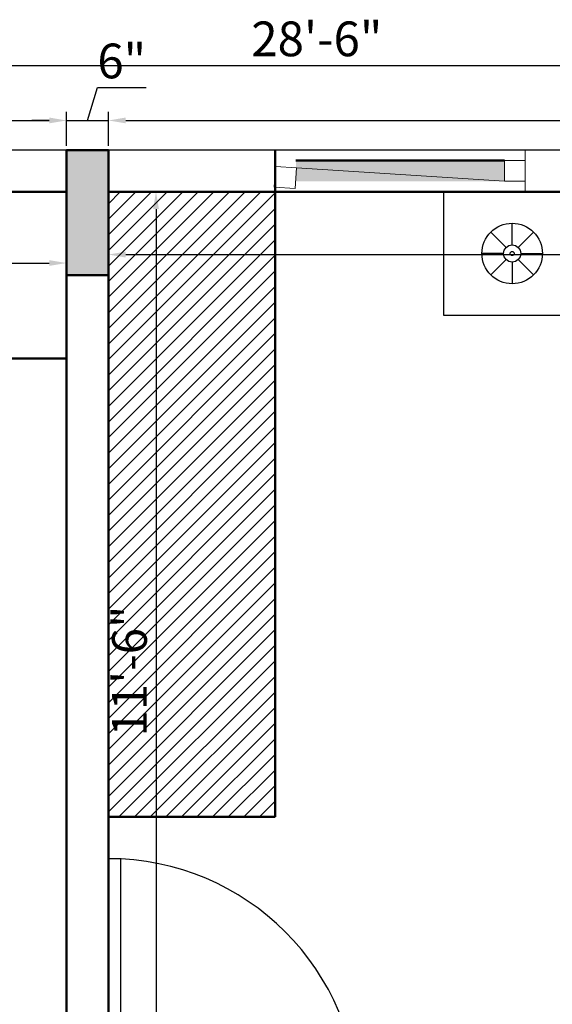
# Model space of a CAD drawing. Units: inches. Extents: x 3064 to 19385, y 846 to 15425.
# Tile 87 of 108: x 7228 to 7305, y 1273 to 1415. Entities that reach past the tile are written whole.
import ezdxf

# ---------------------------------------------------------------- set-up
doc = ezdxf.new("R2010")
doc.units = ezdxf.units.IN
for name, color, linetype, lineweight in [('A-ANNO-DIMS', 2, 'Continuous', 18), ('A-COLS', 1, 'Continuous', 35), ('A-DOOR', 3, 'Continuous', 25), ('A-FLOR-FIXT', 9, 'Continuous', 18), ('A-FURN-PATT', 252, 'Continuous', 13), ('A-GLAZ', 4, 'Continuous', 18), ('A-WALL', 7, 'Continuous', 50), ('C-PROP', 6, 'Continuous', 25)]:
    doc.layers.add(name, color=color, linetype=linetype, lineweight=lineweight)
doc.layers.add('BLOCK', color=6, linetype='Continuous')
doc.styles.get("Standard").update_dxf_attribs({"font": 'arial.ttf'})
doc.dimstyles.new('ISO-25', dxfattribs={"dimtxt": 9, "dimasz": 2.5, "dimexe": 1.25, "dimexo": 0.625, "dimtad": 1, "dimdec": 1, "dimlunit": 3, "dimtxsty": 'Standard', "dimcen": 2.5, "dimadec": 0, "dimazin": 0, "dimtfac": 1, "dimtdec": 1, "dimtmove": 0, "dimatfit": 3, "dimfxl": 1, "dimarcsym": 0})

# ---------------------------------------------------------------- blocks, each defined once
blk = doc.blocks.new('*U3')
for p, q in [((0, 0), (0, -6)), ((36, 0), (36, -6))]:
    blk.add_line(p, q)
blk.add_lwpolyline([(0, 0), (0, 36), (1.75, 36), (1.75, 0)], close=True)
blk.add_arc((0, 0), 36, 0, 90)
blk = doc.blocks.new('*D292')
at = {"layer": 'A-ANNO-DIMS', "color": 0, "lineweight": -2, "transparency": 16777216}
for p, q in [((7105.71, 1396.96), (7105.71, 1401.84)), ((7234.71, 1396.96), (7234.71, 1401.84)), ((7108.21, 1400.59), (7232.21, 1400.59))]:
    blk.add_line(p, q, dxfattribs=at)
at = {"layer": 'A-ANNO-DIMS', "color": 0, "transparency": 16777216}
for points in [[(7108.21, 1401.01), (7108.21, 1400.18), (7105.71, 1400.59)], [(7232.21, 1401.01), (7232.21, 1400.18), (7234.71, 1400.59)]]:
    blk.add_solid(points, dxfattribs=at)
at = {"layer": 'Defpoints', "color": 0, "transparency": 16777216}
for p in [(7234.71, 1400.59), (7105.71, 1396.34), (7234.71, 1396.34)]:
    blk.add_point(p, dxfattribs=at)
at = {"layer": 'A-ANNO-DIMS', "color": 0, "transparency": 16777216, "insert": (7170.21, 1403.77), "char_height": 5, "attachment_point": 5}
blk.add_mtext('10\'-9"', dxfattribs=at)
blk = doc.blocks.new('*D293')
at = {"layer": 'A-ANNO-DIMS', "color": 0, "lineweight": -2, "transparency": 16777216}
for p, q in [((7237.71, 1400.59), (7239.13, 1405.33)), ((7239.13, 1405.33), (7246.15, 1405.33)), ((7234.71, 1396.96), (7234.71, 1401.84)), ((7240.71, 1396.96), (7240.71, 1401.84)), ((7232.21, 1400.59), (7229.71, 1400.59)), ((7234.71, 1400.59), (7240.71, 1400.59)), ((7234.71, 1400.59), (7240.71, 1400.59)), ((7243.21, 1400.59), (7245.71, 1400.59))]:
    blk.add_line(p, q, dxfattribs=at)
at = {"layer": 'A-ANNO-DIMS', "color": 0, "transparency": 16777216}
for points in [[(7232.21, 1401.01), (7232.21, 1400.18), (7234.71, 1400.59)], [(7243.21, 1401.01), (7243.21, 1400.18), (7240.71, 1400.59)]]:
    blk.add_solid(points, dxfattribs=at)
at = {"layer": 'Defpoints', "color": 0, "transparency": 16777216}
for p in [(7240.71, 1400.59), (7234.71, 1396.34), (7240.71, 1396.34)]:
    blk.add_point(p, dxfattribs=at)
at = {"layer": 'A-ANNO-DIMS', "color": 0, "transparency": 16777216, "insert": (7242.64, 1408.51), "char_height": 5, "attachment_point": 5}
blk.add_mtext('6"', dxfattribs=at)
blk = doc.blocks.new('*D294')
at = {"layer": 'A-ANNO-DIMS', "color": 0, "lineweight": -2, "transparency": 16777216}
for p, q in [((7240.71, 1396.96), (7240.71, 1401.84)), ((7435.71, 1396.96), (7435.71, 1401.84)), ((7243.21, 1400.59), (7433.21, 1400.59))]:
    blk.add_line(p, q, dxfattribs=at)
at = {"layer": 'A-ANNO-DIMS', "color": 0, "transparency": 16777216}
for points in [[(7243.21, 1401.01), (7243.21, 1400.18), (7240.71, 1400.59)], [(7433.21, 1401.01), (7433.21, 1400.18), (7435.71, 1400.59)]]:
    blk.add_solid(points, dxfattribs=at)
at = {"layer": 'Defpoints', "color": 0, "transparency": 16777216}
for p in [(7435.71, 1400.59), (7240.71, 1396.34), (7435.71, 1396.34)]:
    blk.add_point(p, dxfattribs=at)
at = {"layer": 'A-ANNO-DIMS', "color": 0, "transparency": 16777216, "insert": (7338.21, 1403.77), "char_height": 5, "attachment_point": 5}
blk.add_mtext('16\'-3"', dxfattribs=at)
blk = doc.blocks.new('*D315')
at = {"layer": 'A-ANNO-DIMS', "color": 0, "lineweight": -2, "transparency": 16777216}
for p, q in [((7099.71, 1396.96), (7099.71, 1409.76)), ((7441.71, 1396.96), (7441.71, 1409.76)), ((7102.21, 1408.51), (7439.21, 1408.51))]:
    blk.add_line(p, q, dxfattribs=at)
at = {"layer": 'A-ANNO-DIMS', "color": 0, "transparency": 16777216}
for points in [[(7102.21, 1408.93), (7102.21, 1408.1), (7099.71, 1408.51)], [(7439.21, 1408.93), (7439.21, 1408.1), (7441.71, 1408.51)]]:
    blk.add_solid(points, dxfattribs=at)
at = {"layer": 'Defpoints', "color": 0, "transparency": 16777216}
for p in [(7441.71, 1408.51), (7099.71, 1396.34), (7441.71, 1396.34)]:
    blk.add_point(p, dxfattribs=at)
at = {"layer": 'A-ANNO-DIMS', "color": 0, "transparency": 16777216, "insert": (7270.71, 1411.69), "char_height": 5, "attachment_point": 5}
blk.add_mtext('28\'-6"', dxfattribs=at)
blk = doc.blocks.new('*D288')
at = {"layer": 'A-ANNO-DIMS', "color": 0, "lineweight": -2, "transparency": 16777216}
for p, q in [((7105.71, 1389.71), (7105.71, 1378.82)), ((7234.71, 1389.71), (7234.71, 1378.82)), ((7108.21, 1380.07), (7232.21, 1380.07))]:
    blk.add_line(p, q, dxfattribs=at)
at = {"layer": 'A-ANNO-DIMS', "color": 0, "transparency": 16777216}
for points in [[(7108.21, 1380.49), (7108.21, 1379.66), (7105.71, 1380.07)], [(7232.21, 1380.49), (7232.21, 1379.66), (7234.71, 1380.07)]]:
    blk.add_solid(points, dxfattribs=at)
at = {"layer": 'Defpoints', "color": 0, "transparency": 16777216}
for p in [(7105.71, 1390.34), (7234.71, 1390.34), (7234.71, 1380.07)]:
    blk.add_point(p, dxfattribs=at)
at = {"layer": 'A-ANNO-DIMS', "color": 0, "transparency": 16777216, "insert": (7170.21, 1383.25), "char_height": 5, "attachment_point": 5}
blk.add_mtext('10\'-9"', dxfattribs=at)
blk = doc.blocks.new('*D290')
at = {"layer": 'A-ANNO-DIMS', "color": 0, "lineweight": -2, "transparency": 16777216}
for p, q in [((7240.71, 1389.71), (7240.71, 1380.04)), ((7435.71, 1389.71), (7435.71, 1380.04)), ((7243.21, 1381.29), (7433.21, 1381.29))]:
    blk.add_line(p, q, dxfattribs=at)
at = {"layer": 'A-ANNO-DIMS', "color": 0, "transparency": 16777216}
for points in [[(7243.21, 1381.71), (7243.21, 1380.87), (7240.71, 1381.29)], [(7433.21, 1381.71), (7433.21, 1380.87), (7435.71, 1381.29)]]:
    blk.add_solid(points, dxfattribs=at)
at = {"layer": 'Defpoints', "color": 0, "transparency": 16777216}
for p in [(7240.71, 1390.34), (7435.71, 1390.34), (7435.71, 1381.29)]:
    blk.add_point(p, dxfattribs=at)
at = {"layer": 'A-ANNO-DIMS', "color": 0, "transparency": 16777216, "insert": (7338.21, 1384.47), "char_height": 5, "attachment_point": 5}
blk.add_mtext('16\'-3"', dxfattribs=at)
blk = doc.blocks.new('*D275')
at = {"layer": 'A-ANNO-DIMS', "color": 0, "lineweight": -2, "transparency": 16777216}
for p, q in [((7241.33, 1390.34), (7248.82, 1390.34)), ((7247.57, 1387.84), (7247.57, 1254.84)), ((7241.33, 1252.34), (7248.82, 1252.34))]:
    blk.add_line(p, q, dxfattribs=at)
at = {"layer": 'A-ANNO-DIMS', "color": 0, "transparency": 16777216}
for points in [[(7247.15, 1387.84), (7247.99, 1387.84), (7247.57, 1390.34)], [(7247.15, 1254.84), (7247.99, 1254.84), (7247.57, 1252.34)]]:
    blk.add_solid(points, dxfattribs=at)
at = {"layer": 'Defpoints', "color": 0, "transparency": 16777216}
for p in [(7240.71, 1390.34), (7240.71, 1252.34), (7247.57, 1252.34)]:
    blk.add_point(p, dxfattribs=at)
at = {"layer": 'A-ANNO-DIMS', "color": 0, "transparency": 16777216, "insert": (7244.39, 1321.34), "char_height": 5, "attachment_point": 5, "rotation": 90}
blk.add_mtext('11\'-6"', dxfattribs=at)
blk = doc.blocks.new('A$C52E67D0D')
at = {"layer": 'BLOCK'}
for p, q in [((250.5, 1605.5), (250.5, 1684.7)), ((228.3, 1596.3), (172.3, 1652.3)), ((272.7, 1596.3), (328.7, 1652.3)), ((219.1, 1574.1), (139.9, 1574.1)), ((228.3, 1551.9), (172.3, 1495.9)), ((272.7, 1551.9), (328.7, 1495.9)), ((281.9, 1574.1), (361.1, 1574.1)), ((250.5, 1542.8), (250.5, 1463.5))]:
    blk.add_line(p, q, dxfattribs=at)
blk.add_lwpolyline([(501, 1348.6), (501, 1799.6), (0, 1799.6), (0, 1348.6)], close=True, dxfattribs=at)
for radius in [110.6, 31.4, 7.46]:
    blk.add_circle((250.5, 1574.1), radius, dxfattribs=at)
blk = doc.blocks.new('WIN-900')
blk.add_line((0, 0), (30, 0))
blk.add_lwpolyline([(30, 0), (30, 3), (33, 3), (33, 0)], close=True)

msp = doc.modelspace()

# ---------------------------------------------------------------- hatches: boundary and pattern name
at = {"layer": 'A-COLS'}
h = msp.add_hatch(color=256, dxfattribs=at)
h.dxf.hatch_style = 1
h.paths.add_polyline_path([(7234.71, 1378.34), (7240.71, 1378.34), (7240.71, 1396.34), (7234.71, 1396.34)])
at = {"layer": 'A-FURN-PATT'}
h = msp.add_hatch(dxfattribs=at)
h.set_pattern_fill('ANSI31', color=256, scale=0.5)
h.set_pattern_definition([(45, (1784.0376, -1e-11), (-1.122532, 1.122532), [])])
h.paths.add_polyline_path([(7264.71, 1390.34), (7240.71, 1390.34), (7240.71, 1378.34), (7240.71, 1300.34), (7264.71, 1300.34)])
at = {"layer": 'A-GLAZ'}
h = msp.add_hatch(color=256, dxfattribs=at)
h.dxf.hatch_style = 1
h.paths.add_polyline_path([(7297.71, 1394.84), (7267.71, 1394.84), (7267.71, 1391.84), (7297.71, 1391.84)])

# ---------------------------------------------------------------- linework, layer by layer
msp.add_line((7300.71, 1396.34), (7300.71, 1390.34), dxfattribs=at)
msp.add_lwpolyline([(7300.71, 1391.84), (7297.71, 1391.84), (7297.71, 1394.84), (7300.71, 1394.84)], close=True, dxfattribs=at)
at = {"layer": 'A-WALL'}
for p, q in [((7264.71, 1396.34), (7264.71, 1390.34)), ((7267.71, 1394.84), (7297.71, 1394.84)), ((7234.71, 1390.34), (7105.71, 1390.34)), ((7234.71, 1390.34), (7234.71, 1252.34)), ((7435.71, 1390.34), (7240.71, 1390.34)), ((7240.71, 1390.34), (7240.71, 1252.34)), ((7264.71, 1390.34), (7264.71, 1300.34)), ((7234.71, 1366.34), (7129.71, 1366.34)), ((7264.71, 1300.34), (7240.71, 1300.34))]:
    msp.add_line(p, q, dxfattribs=at)
msp.add_lwpolyline([(7240.71, 1378.34), (7240.71, 1396.34), (7234.71, 1396.34), (7234.71, 1378.34)], close=True, dxfattribs=at)
at = {"layer": 'C-PROP'}
msp.add_line((7441.71, 1396.34), (7099.71, 1396.34), dxfattribs=at)

# ---------------------------------------------------------------- block references
at = {"layer": 'A-DOOR'}
msp.add_blockref('*U3', (7240.71, 1258.34), dxfattribs=at)
at = {"layer": 'A-FLOR-FIXT', "xscale": 0.039370099999992, "yscale": 0.039370099999992, "zscale": 0.039370099999992}
msp.add_blockref('A$C52E67D0D', (7288.95, 1319.47), dxfattribs=at)
at = {"layer": 'A-GLAZ', "rotation": 176.304779468011}
msp.add_blockref('WIN-900', (7297.71, 1391.84), dxfattribs=at)

# ---------------------------------------------------------------- dimensions: what is measured, and where the dimension line sits
at = {"layer": 'A-ANNO-DIMS'}
for base, p1, p2, override, picture, middle in [((7441.71, 1408.51), (7099.71, 1396.34), (7441.71, 1396.34), {"dimtxt": 5, "dimclrd": 0, "dimclre": 0, "dimclrt": 0}, '*D315', (7270.71, 1411.69)), ((7240.71, 1400.59), (7234.71, 1396.34), (7240.71, 1396.34), {"dimtxt": 5, "dimclrd": 0, "dimclre": 0, "dimclrt": 0, "dimtmove": 1}, '*D293', (7239.75, 1408.51)), ((7234.71, 1400.59), (7105.71, 1396.34), (7234.71, 1396.34), {"dimtxt": 5, "dimclrd": 0, "dimclre": 0, "dimclrt": 0, "dimtmove": 1}, '*D292', (7170.21, 1403.77)), ((7435.71, 1400.59), (7240.71, 1396.34), (7435.71, 1396.34), {"dimtxt": 5, "dimclrd": 0, "dimclre": 0, "dimclrt": 0, "dimtmove": 1}, '*D294', (7338.21, 1403.77)), ((7234.71, 1380.07), (7105.71, 1390.34), (7234.71, 1390.34), {"dimtxt": 5, "dimclrd": 0, "dimclre": 0, "dimclrt": 0}, '*D288', (7170.21, 1383.25)), ((7435.71, 1381.29), (7240.71, 1390.34), (7435.71, 1390.34), {"dimtxt": 5, "dimclrd": 0, "dimclre": 0, "dimclrt": 0}, '*D290', (7338.21, 1384.47))]:
    dim = msp.add_linear_dim(base=base, p1=p1, p2=p2, dimstyle='ISO-25', override=override, dxfattribs=at)
    dim.commit()
    dim.dimension.update_dxf_attribs({"geometry": picture, "text_midpoint": middle})
dim = msp.add_linear_dim(base=(7247.57, 1252.34), p1=(7240.71, 1390.34), p2=(7240.71, 1252.34), angle=90, dimstyle='ISO-25', override={"dimtxt": 5, "dimclrd": 0, "dimclre": 0, "dimclrt": 0}, dxfattribs=at)
dim.commit()
dim.dimension.update_dxf_attribs({"geometry": '*D275', "text_midpoint": (7244.39, 1321.34)})

doc.saveas('drawing.dxf')
